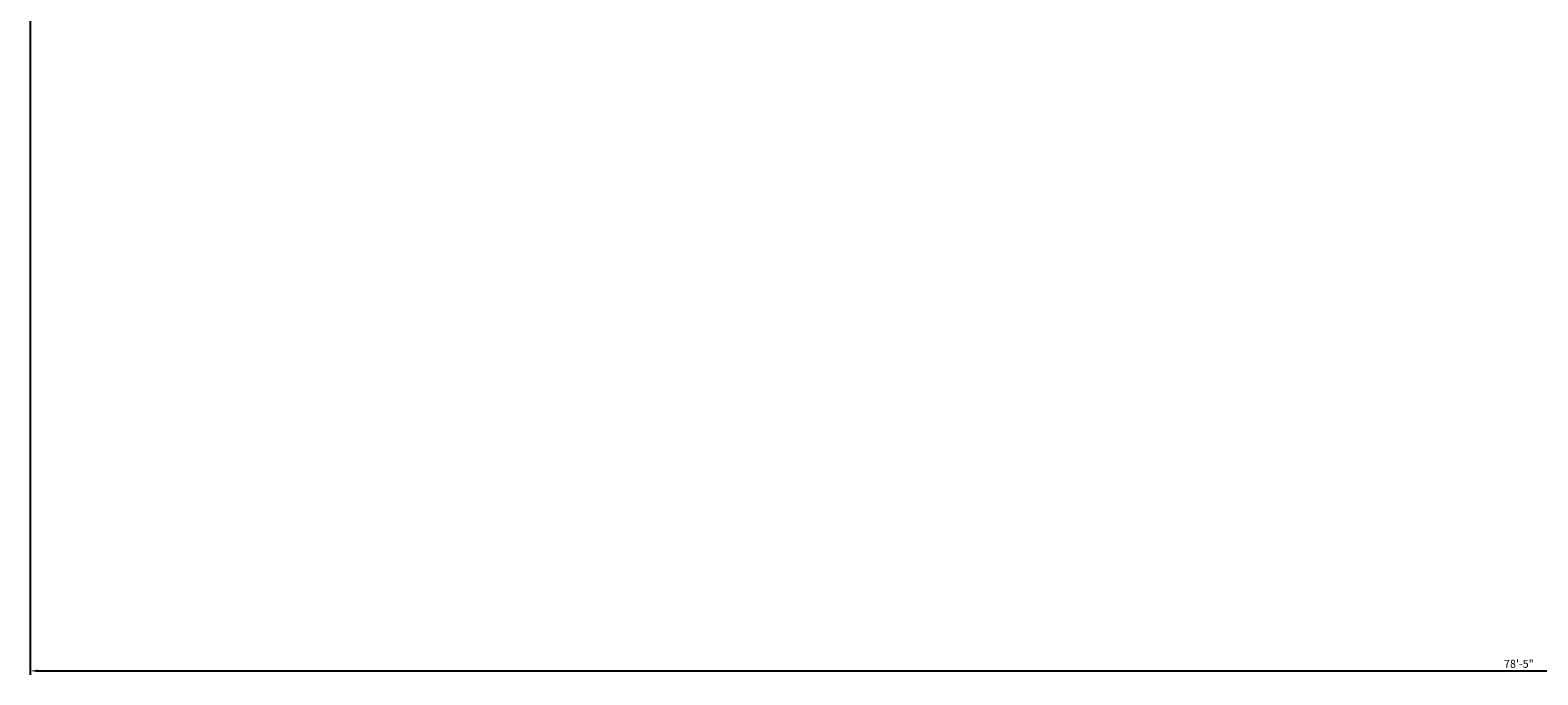
# Model space of a CAD drawing. Units: inches. Extents: x 7028582 to 7030319, y 63109697 to 63111305.
# Tile 3 of 18: x 7029235 to 7029711, y 63109697 to 63109901. Entities that reach past the tile are written whole.
import ezdxf

# ---------------------------------------------------------------- set-up
doc = ezdxf.new("R2010")
doc.units = ezdxf.units.IN
doc.layers.add('C-ANNO-DIMS', color=7, linetype='Continuous', lineweight=18)
doc.styles.get("Standard").update_dxf_attribs({"font": 'arial.ttf'})
doc.dimstyles.new('ISO-25', dxfattribs={"dimtxt": 2.5, "dimasz": 2.5, "dimexe": 1.25, "dimexo": 0.625, "dimtad": 1, "dimlunit": 4, "dimtxsty": 'Standard', "dimcen": 2.5, "dimadec": 0, "dimazin": 0, "dimtfac": 1, "dimtmove": 0, "dimatfit": 3, "dimfxl": 1, "dimarcsym": 0})

# ---------------------------------------------------------------- blocks, each defined once
blk = doc.blocks.new('*D99')
at = {"layer": 'C-ANNO-DIMS', "color": 0, "lineweight": -2, "transparency": 16777216}
for p, q in [((7029234.71, 63109965.93), (7029234.71, 63109697.14)), ((7030175.71, 63109965.93), (7030175.71, 63109697.14)), ((7029237.21, 63109698.39), (7030173.21, 63109698.39))]:
    blk.add_line(p, q, dxfattribs=at)
at = {"layer": 'C-ANNO-DIMS', "color": 0, "lineweight": 100, "transparency": 16777216}
for points in [[(7029237.21, 63109698.8), (7029237.21, 63109697.97), (7029234.71, 63109698.39)], [(7030173.21, 63109698.8), (7030173.21, 63109697.97), (7030175.71, 63109698.39)]]:
    blk.add_solid(points, dxfattribs=at)
at = {"layer": 'Defpoints', "color": 0, "lineweight": 100, "transparency": 16777216}
for p in [(7029234.71, 63109966.56), (7030175.71, 63109966.56), (7030175.71, 63109698.39)]:
    blk.add_point(p, dxfattribs=at)
at = {"layer": 'C-ANNO-DIMS', "color": 0, "transparency": 16777216, "insert": (7029705.21, 63109700.29), "char_height": 2.5, "attachment_point": 5}
blk.add_mtext('78\'-5"', dxfattribs=at)

msp = doc.modelspace()

# ---------------------------------------------------------------- dimensions: what is measured, and where the dimension line sits
at = {"layer": 'C-ANNO-DIMS'}
dim = msp.add_linear_dim(base=(7030175.705, 63109698.385), p1=(7029234.705, 63109966.557), p2=(7030175.705, 63109966.557), dimstyle='ISO-25', override={"dimdec": 1, "dimlfac": 1, "dimrnd": 0, "dimzin": 1, "dimdsep": 46, "dimlunit": 4, "dimfrac": 2}, dxfattribs=at)
dim.commit()
dim.dimension.update_dxf_attribs({"geometry": '*D99', "text_midpoint": (7029705.205, 63109700.287)})

doc.saveas('drawing.dxf')
